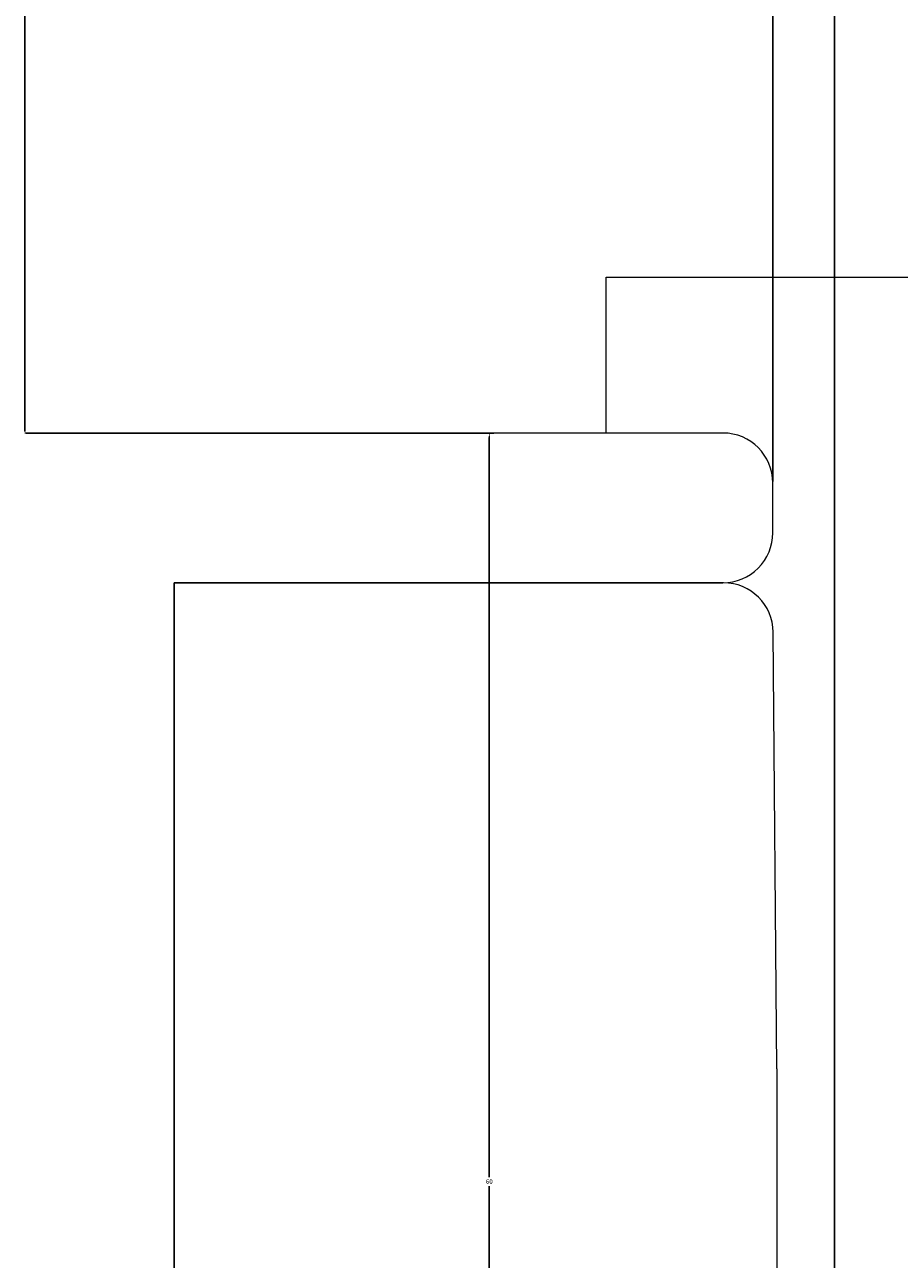
# Model space of a CAD drawing. Units: inches. Extents: x 2231 to 2461, y 2045 to 2455.
# Tile 42 of 95: x 2262 to 2297, y 2222 to 2271. Entities that reach past the tile are written whole.
import ezdxf

# ---------------------------------------------------------------- set-up
doc = ezdxf.new("R2010")
doc.units = ezdxf.units.IN
doc.layers.add('A-ANNO-DIMS', color=2, linetype='Continuous', lineweight=18)
doc.layers.add('A-FURN', color=9, linetype='Continuous', lineweight=18)
doc.styles.get("Standard").update_dxf_attribs({"font": 'arial.ttf'})
doc.dimstyles.get("Standard").update_dxf_attribs({"dimtxt": 0.18, "dimasz": 0.18, "dimexe": 0.18, "dimexo": 0.0625, "dimgap": 0.09, "dimtad": 0, "dimtih": 1, "dimtoh": 1, "dimdec": 4, "dimzin": 0, "dimdsep": 46, "dimtxsty": 'Standard', "dimcen": 0.09, "dimadec": 0, "dimazin": 0, "dimtfac": 1, "dimtdec": 4, "dimtofl": 0, "dimtmove": 0, "dimatfit": 3, "dimfxl": 1, "dimtolj": 1, "dimtzin": 0, "dimarcsym": 0})

# ---------------------------------------------------------------- blocks, each defined once
blk = doc.blocks.new('*D47')
at = {"layer": 'A-ANNO-DIMS', "color": 0, "lineweight": -2, "transparency": 16777216}
for p, q in [((2258.794, 2182.895), (2258.794, 2454.645)), ((2258.974, 2454.465), (2276.575, 2454.465)), ((2294.614, 2454.465), (2277.012, 2454.465)), ((2294.794, 2182.895), (2294.794, 2454.645))]:
    blk.add_line(p, q, dxfattribs=at)
at = {"layer": 'A-ANNO-DIMS', "color": 0, "transparency": 16777216}
for points in [[(2258.974, 2454.495), (2258.974, 2454.435), (2258.794, 2454.465)], [(2294.614, 2454.495), (2294.614, 2454.435), (2294.794, 2454.465)]]:
    blk.add_solid(points, dxfattribs=at)
at = {"layer": 'Defpoints', "color": 0, "transparency": 16777216}
for p in [(2294.794, 2454.465), (2258.794, 2182.833), (2294.794, 2182.833)]:
    blk.add_point(p, dxfattribs=at)
at = {"layer": 'A-ANNO-DIMS', "color": 0, "transparency": 16777216, "insert": (2276.794, 2454.465), "char_height": 0.18, "attachment_point": 5}
blk.add_mtext('\\A1;36', dxfattribs=at)
blk = doc.blocks.new('*D51')
at = {"layer": 'A-ANNO-DIMS', "color": 0, "lineweight": -2, "transparency": 16777216}
for p, q in [((2258.794, 2306.77), (2258.794, 2044.803)), ((2330.794, 2306.77), (2330.794, 2044.803)), ((2258.974, 2044.983), (2294.576, 2044.983)), ((2330.614, 2044.983), (2295.011, 2044.983))]:
    blk.add_line(p, q, dxfattribs=at)
at = {"layer": 'A-ANNO-DIMS', "color": 0, "transparency": 16777216}
for points in [[(2258.974, 2045.013), (2258.974, 2044.953), (2258.794, 2044.983)], [(2330.614, 2045.013), (2330.614, 2044.953), (2330.794, 2044.983)]]:
    blk.add_solid(points, dxfattribs=at)
at = {"layer": 'Defpoints', "color": 0, "transparency": 16777216}
for p in [(2258.794, 2306.833), (2330.794, 2306.833), (2330.794, 2044.983)]:
    blk.add_point(p, dxfattribs=at)
at = {"layer": 'A-ANNO-DIMS', "color": 0, "transparency": 16777216, "insert": (2294.794, 2044.983), "char_height": 0.18, "attachment_point": 5}
blk.add_mtext('\\A1;72', dxfattribs=at)
blk = doc.blocks.new('*D62')
at = {"layer": 'A-ANNO-DIMS', "color": 0, "lineweight": -2, "transparency": 16777216}
for p, q in [((2262.321, 2255.176), (2262.321, 2454.645)), ((2262.501, 2454.465), (2277.102, 2454.465)), ((2292.141, 2454.465), (2277.539, 2454.465)), ((2292.321, 2253.176), (2292.321, 2454.645))]:
    blk.add_line(p, q, dxfattribs=at)
at = {"layer": 'A-ANNO-DIMS', "color": 0, "transparency": 16777216}
for points in [[(2262.501, 2454.495), (2262.501, 2454.435), (2262.321, 2454.465)], [(2292.141, 2454.495), (2292.141, 2454.435), (2292.321, 2454.465)]]:
    blk.add_solid(points, dxfattribs=at)
at = {"layer": 'Defpoints', "color": 0, "transparency": 16777216}
for p in [(2292.321, 2454.465), (2262.321, 2255.114), (2292.321, 2253.114)]:
    blk.add_point(p, dxfattribs=at)
at = {"layer": 'A-ANNO-DIMS', "color": 0, "transparency": 16777216, "insert": (2277.321, 2454.465), "char_height": 0.18, "attachment_point": 5}
blk.add_mtext('\\A1;30', dxfattribs=at)
blk = doc.blocks.new('*D63')
at = {"layer": 'A-ANNO-DIMS', "color": 0, "lineweight": -2, "transparency": 16777216}
for p, q in [((2262.383, 2255.114), (2281.133, 2255.114)), ((2280.953, 2254.934), (2280.953, 2225.296)), ((2280.953, 2195.294), (2280.953, 2224.932)), ((2262.383, 2195.114), (2281.133, 2195.114))]:
    blk.add_line(p, q, dxfattribs=at)
at = {"layer": 'A-ANNO-DIMS', "color": 0, "transparency": 16777216}
for points in [[(2280.923, 2254.934), (2280.983, 2254.934), (2280.953, 2255.114)], [(2280.923, 2195.294), (2280.983, 2195.294), (2280.953, 2195.114)]]:
    blk.add_solid(points, dxfattribs=at)
at = {"layer": 'Defpoints', "color": 0, "transparency": 16777216}
for p in [(2262.321, 2255.114), (2262.321, 2195.114), (2280.953, 2195.114)]:
    blk.add_point(p, dxfattribs=at)
at = {"layer": 'A-ANNO-DIMS', "color": 0, "transparency": 16777216, "insert": (2280.953, 2225.114), "char_height": 0.18, "attachment_point": 5}
blk.add_mtext('\\A1;60', dxfattribs=at)

msp = doc.modelspace()

# ---------------------------------------------------------------- linework, layer by layer
at = {"layer": 'A-FURN'}
for p, q in [((2268.3207, 2255.1137), (2262.3207, 2255.1137)), ((2290.3207, 2255.1137), (2268.3207, 2255.1137)), ((2290.3368, 2249.1137), (2268.3207, 2249.1137)), ((2268.3207, 2249.1137), (2268.3207, 2201.1137)), ((2292.4784, 2229.6377), (2292.3368, 2247.1299))]:
    msp.add_line(p, q, dxfattribs=at)
for points in [[(2285.6353, 2255.1137), (2285.6353, 2261.3584), (2340.6673, 2261.3584), (2340.6673, 2189.3477), (2285.6353, 2189.3477), (2285.6353, 2195.1137)], [(2268.3207, 2210.1618), (2268.3207, 2229.6377)], [(2292.4784, 2229.6377), (2292.4784, 2210.1618)]]:
    msp.add_lwpolyline(points, dxfattribs=at)
msp.add_lwpolyline([(2268.3207, 2229.6377), (2268.3207, 2249.1137), (2290.3207, 2249.1137, 0.4142136), (2292.3207, 2251.1137), (2292.3207, 2253.1137)], format="xyb", dxfattribs=at)
for centre, start in [((2290.3207, 2253.1137), 0), ((2290.3368, 2247.1137), 0.46404)]:
    msp.add_arc(centre, 2, start, 90, dxfattribs=at)

# ---------------------------------------------------------------- dimensions: what is measured, and where the dimension line sits
at = {"layer": 'A-ANNO-DIMS'}
for base, p1, p2, picture, middle in [((2294.7935, 2454.4653), (2258.7935, 2182.8328), (2294.7935, 2182.8328), '*D47', (2276.7935, 2454.4653)), ((2292.3207, 2454.4653), (2262.3207, 2255.1137), (2292.3207, 2253.1137), '*D62', (2277.3207, 2454.4653)), ((2330.7935, 2044.9825), (2258.7935, 2306.8328), (2330.7935, 2306.8328), '*D51', (2294.7935, 2044.9825))]:
    dim = msp.add_linear_dim(base=base, p1=p1, p2=p2, dimstyle='Standard', override={"dimdec": 0, "dimlfac": 1, "dimrnd": 0, "dimzin": 0, "dimdsep": 46, "dimlunit": 2}, dxfattribs=at)
    dim.commit()
    dim.dimension.update_dxf_attribs({"geometry": picture, "text_midpoint": middle})
dim = msp.add_linear_dim(base=(2280.9532, 2195.1137), p1=(2262.3207, 2255.1137), p2=(2262.3207, 2195.1137), angle=270, dimstyle='Standard', override={"dimdec": 0, "dimlfac": 1, "dimrnd": 0, "dimzin": 0, "dimdsep": 46, "dimlunit": 2}, dxfattribs=at)
dim.commit()
dim.dimension.update_dxf_attribs({"geometry": '*D63', "text_midpoint": (2280.9532, 2225.1137)})

doc.saveas('drawing.dxf')
